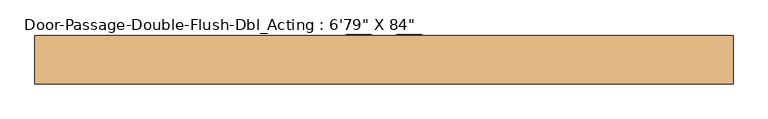
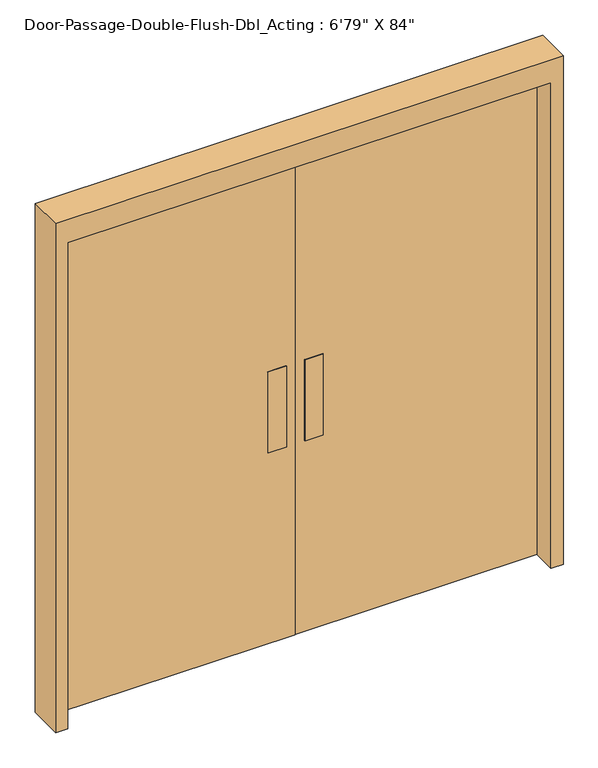
"""IFC4 building model written with IfcOpenShell, lengths in millimetres: door geometry."""

from ifc_helpers import new_model, si_unit, frame, origin, origin_with_axes, place, context, project, spatial, polyline, outline, extrude, source, transform, mapped, element, save


def door_2c854dd0(model_context):
    return source(origin(), model_context, "Body", "SweptSolid", [
        extrude(outline(polyline([(-38.1, 47.625), (-114.3, 47.625), (-114.3, 50.8), (-38.1, 50.8), (-38.1, 47.625)])), frame((0.0, 0.0, 838.2), z_axis=(0.0, 0.0, 1.0), x_axis=(1.0, 0.0, 0.0)), (0.0, 0.0, 1.0), 355.6),
        extrude(outline(polyline([(-38.1, 98.425), (-38.1, 95.25), (-114.3, 95.25), (-114.3, 98.425), (-38.1, 98.425)])), frame((0.0, 0.0, 838.2), z_axis=(0.0, 0.0, 1.0), x_axis=(1.0, 0.0, 0.0)), (0.0, 0.0, 1.0), 355.6),
        extrude(outline(polyline([(38.1, 47.625), (38.1, 50.8), (114.3, 50.8), (114.3, 47.625), (38.1, 47.625)])), frame((0.0, 0.0, 838.2), z_axis=(0.0, 0.0, 1.0), x_axis=(1.0, 0.0, 0.0)), (0.0, 0.0, 1.0), 355.6),
        extrude(outline(polyline([(38.1, 98.425), (114.3, 98.425), (114.3, 95.25), (38.1, 95.25), (38.1, 98.425)])), frame((0.0, 0.0, 838.2), z_axis=(0.0, 0.0, 1.0), x_axis=(1.0, 0.0, 0.0)), (0.0, 0.0, 1.0), 355.6),
        extrude(outline(polyline([(1003.3, 50.8), (1.5875, 50.8), (1.5875, 82.55), (1003.3, 82.55), (1003.3, 50.8)])), origin_with_axes(), (0.0, 0.0, 1.0), 2133.6),
        extrude(outline(polyline([(-1.5875, 50.8), (-1003.3, 50.8), (-1003.3, 82.55), (-1.5875, 82.55), (-1.5875, 50.8)])), origin_with_axes(), (0.0, 0.0, 1.0), 2133.6),
        extrude(outline(polyline([(0.0, 1003.3), (0.0, 1054.1), (2235.2, 1054.1), (2235.2, -1054.1), (0.0, -1054.1), (0.0, -1003.3), (2133.6, -1003.3), (2133.6, 1003.3), (0.0, 1003.3)])), frame((0.0, -50.8, 0.0), z_axis=(0.0, 1.0, 0.0), x_axis=(0.0, 0.0, 1.0)), (0.0, 0.0, 1.0), 146.05),
    ])


if __name__ == "__main__":
    model = new_model("IFC4")
    model_context = context("Model", 3, world=origin())
    ifc_project = project(units=[si_unit("LENGTHUNIT", "METRE", prefix="MILLI")], contexts=[model_context])
    site = spatial("IfcSite", under=ifc_project)
    building = spatial("IfcBuilding", under=site)
    placement = place(None, origin())
    door_shape = door_2c854dd0(model_context)
    element("IfcDoor", 1, ObjectType="Door-Passage-Double-Flush-Dbl_Acting : 6'79\" X 84\"", at=placement, inside=building, context=model_context, shape_type="MappedRepresentation", body=[
        mapped(door_shape, transform((0.0, 0.0, 0.0), x_axis=(1.0, 0.0, 0.0), y_axis=(0.0, 1.0, 0.0), z_axis=(0.0, 0.0, 1.0))),
    ])
    save(model, "model.ifc")

# Revit data of these elements
# Type "Door-Passage-Double-Flush-Dbl_Acting : 6'79\" X 84\""
#   Type Mark = "17"
#   Assembly Code = "B2030200"
#   Analytic Construction = "Metal"
#   W = 3' - 3 1/2"
#   Thickness = 0' - 1 3/4"
#   Thermal Resistance (R) = 1.5338 (h·ft²·°F)/BTU
#   Swing Angle [instance default] = 90.00°
#   Strike Height = 3' - 4"
#   Single Panel Width = 3' - 3 1/2"
#   Rough Width [instance default] = 6' - 11"
#   Rough Height [instance default] = 7' - 4"
#   MF Opening Height [instance default] = 0' - 4"
#   MF Opening Width [instance default] = 0' - 4"
#   Inset Calculate [instance default] = 0' - 4"
#   Masonry Inset [instance default] = 0' - 1"
#   Height = 7' - 0"
#   Width = 6' - 7"
#   Heat Transfer Coefficient (U) = 0.6520 BTU/(h·ft²·°F)
#   Masonry Frame Depth = 0' - 5 3/4"
#   Masonry Frame [instance default] = yes
#   Function = 1
#   Dry Wall Frame [instance default] = no
#   Panel Material = Metal - Paint Finish - Brindle
#   Frame Material = Metal - Paint Finish - Grey
#   Door Handle Material = Aluminium
#   Visual Light Transmittance = 0
#   Solar Heat Gain Coefficient = 0
#   Wall Closure = (empty or 0)
# Element 1 (IfcDoor, "Door-Passage-Double-Flush-Dbl_Acting : 6'79\" X 84\"")
#   Materials on its faces: "Aluminium", "Metal - Paint Finish - Brindle", "Metal - Paint Finish - Grey"
# Materials
#   "Metal - Paint Finish - Brindle": class "Paint", colour RGB 164 133 98, transparency 0, Cost = 0
#   "Metal - Paint Finish - Grey": class "Paint", colour RGB 104 104 104, transparency 0, Cost = 0
#   "Aluminium": class "Metal", colour RGB 244 244 244, transparency 0, Description = "Aluminum 6061", Cost = 0
